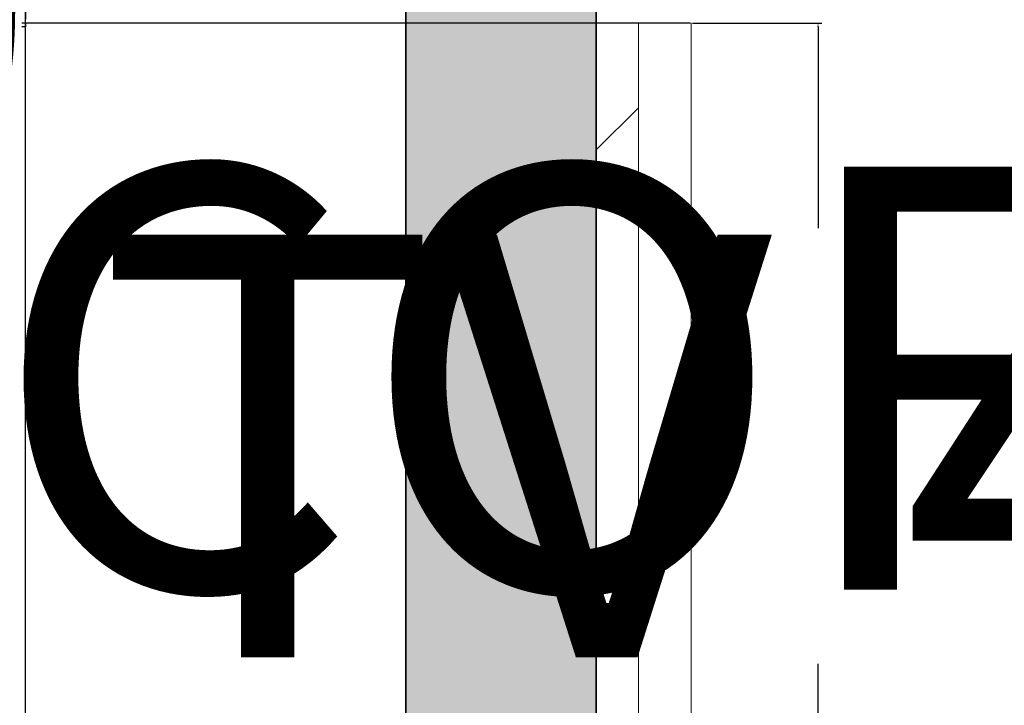
# Model space of a CAD drawing. Units: inches. Extents: x 305 to 776, y 38 to 479.
# Tile 4 of 14: x 372 to 419, y 199 to 231. Entities that reach past the tile are written whole.
import ezdxf

# ---------------------------------------------------------------- set-up
doc = ezdxf.new("R2010")
doc.units = ezdxf.units.IN
doc.header["$MEASUREMENT"] = 0
for name, color, linetype, lineweight in [('A-ANNO-DIMS', 2, 'Continuous', 18), ('A-EQPM', 8, 'Continuous', 18), ('A-WALL', 7, 'Continuous', 35), ('A-WALL-PATT', 252, 'Continuous', 13)]:
    doc.layers.add(name, color=color, linetype=linetype, lineweight=lineweight)
doc.styles.get("Standard").update_dxf_attribs({"font": 'arial.ttf'})
doc.dimstyles.get("Standard").update_dxf_attribs({"dimtxt": 20, "dimasz": 0.18, "dimexe": 0.18, "dimexo": 0.0625, "dimgap": 0.09, "dimtad": 0, "dimtih": 1, "dimtoh": 1, "dimdec": 4, "dimzin": 0, "dimdsep": 46, "dimtxsty": 'Standard', "dimcen": 0.09, "dimadec": 0, "dimazin": 0, "dimtfac": 1, "dimtdec": 4, "dimtofl": 0, "dimtmove": 0, "dimatfit": 3, "dimfxl": 1, "dimtolj": 1, "dimtzin": 0, "dimarcsym": 0})

# ---------------------------------------------------------------- blocks, each defined once
blk = doc.blocks.new('TV')
for p, q in [((722.63, 295.634), (720.13, 295.634)), ((720.13, 295.634), (720.13, 255.634)), ((722.63, 255.634), (722.63, 295.634)), ((720.13, 291.634), (718.13, 289.634)), ((718.13, 289.634), (718.13, 261.634)), ((720.13, 259.634), (718.13, 261.634)), ((720.13, 255.634), (722.63, 255.634))]:
    blk.add_line(p, q)
blk = doc.blocks.new('*D19')
at = {"layer": 'A-ANNO-DIMS', "color": 0, "lineweight": -2, "transparency": 16777216}
for p, q in [((557.633, 250.82), (557.633, 245.977)), ((589.133, 250.82), (589.133, 245.977)), ((557.633, 246.157), (557.453, 246.157)), ((588.953, 246.157), (557.813, 246.157))]:
    blk.add_line(p, q, dxfattribs=at)
at = {"layer": 'A-ANNO-DIMS', "color": 0, "transparency": 16777216}
for points in [[(557.813, 246.187), (557.813, 246.127), (557.633, 246.157)], [(588.953, 246.187), (588.953, 246.127), (589.133, 246.157)]]:
    blk.add_solid(points, dxfattribs=at)
at = {"layer": 'Defpoints', "color": 0, "transparency": 16777216}
for p in [(557.633, 250.882), (589.133, 250.882), (557.633, 246.157)]:
    blk.add_point(p, dxfattribs=at)
at = {"layer": 'A-ANNO-DIMS', "color": 0, "transparency": 16777216, "insert": (463.393, 246.157), "char_height": 20, "attachment_point": 5}
blk.add_mtext('\\A1;DOOR 32 TYP.', dxfattribs=at)
blk = doc.blocks.new('*D37')
at = {"layer": 'A-ANNO-DIMS', "color": 0, "lineweight": -2, "transparency": 16777216}
for p, q in [((476.346, 237.029), (483.222, 237.029)), ((483.042, 236.849), (483.042, 224.939)), ((483.042, 192.153), (483.042, 204.063)), ((476.346, 191.973), (483.222, 191.973))]:
    blk.add_line(p, q, dxfattribs=at)
at = {"layer": 'A-ANNO-DIMS', "color": 0, "transparency": 16777216}
for points in [[(483.012, 236.849), (483.072, 236.849), (483.042, 237.029)], [(483.012, 192.153), (483.072, 192.153), (483.042, 191.973)]]:
    blk.add_solid(points, dxfattribs=at)
at = {"layer": 'Defpoints', "color": 0, "transparency": 16777216}
for p in [(476.283, 237.029), (483.042, 237.029), (476.283, 191.973)]:
    blk.add_point(p, dxfattribs=at)
at = {"layer": 'A-ANNO-DIMS', "color": 0, "transparency": 16777216, "insert": (483.042, 214.501), "char_height": 20, "attachment_point": 5}
blk.add_mtext('\\A1;COFFEE TABLE 45', dxfattribs=at)
blk = doc.blocks.new('*D39')
at = {"layer": 'A-ANNO-DIMS', "color": 0, "lineweight": -2, "transparency": 16777216}
for p, q in [((404.195, 231.292), (410.313, 231.292)), ((410.133, 231.112), (410.133, 221.593)), ((410.133, 191.472), (410.133, 200.99)), ((404.195, 191.292), (410.313, 191.292))]:
    blk.add_line(p, q, dxfattribs=at)
at = {"layer": 'A-ANNO-DIMS', "color": 0, "transparency": 16777216}
for points in [[(410.103, 231.112), (410.163, 231.112), (410.133, 231.292)], [(410.103, 191.472), (410.163, 191.472), (410.133, 191.292)]]:
    blk.add_solid(points, dxfattribs=at)
at = {"layer": 'Defpoints', "color": 0, "transparency": 16777216}
for p in [(404.133, 231.292), (410.133, 231.292), (404.133, 191.292)]:
    blk.add_point(p, dxfattribs=at)
at = {"layer": 'A-ANNO-DIMS', "color": 0, "transparency": 16777216, "insert": (410.133, 211.292), "char_height": 20, "attachment_point": 5}
blk.add_mtext('\\A1;TV 40', dxfattribs=at)
blk = doc.blocks.new('*D46')
at = {"layer": 'A-ANNO-DIMS', "color": 0, "lineweight": -2, "transparency": 16777216}
for p, q in [((390.57, 429.382), (372.451, 429.382)), ((372.631, 429.202), (372.631, 259.69)), ((372.631, 69.562), (372.631, 239.074)), ((390.57, 69.382), (372.451, 69.382))]:
    blk.add_line(p, q, dxfattribs=at)
at = {"layer": 'A-ANNO-DIMS', "color": 0, "transparency": 16777216}
for points in [[(372.601, 429.202), (372.661, 429.202), (372.631, 429.382)], [(372.601, 69.562), (372.661, 69.562), (372.631, 69.382)]]:
    blk.add_solid(points, dxfattribs=at)
at = {"layer": 'Defpoints', "color": 0, "transparency": 16777216}
for p in [(372.631, 429.382), (390.633, 429.382), (390.633, 69.382)]:
    blk.add_point(p, dxfattribs=at)
at = {"layer": 'A-ANNO-DIMS', "color": 0, "transparency": 16777216, "insert": (372.631, 249.382), "char_height": 20, "attachment_point": 5}
blk.add_mtext('\\A1;360', dxfattribs=at)
blk = doc.blocks.new('*D62')
at = {"layer": 'A-ANNO-DIMS', "color": 0, "lineweight": -2, "transparency": 16777216}
for p, q in [((399.633, 336.32), (399.633, 51.201)), ((423.233, 336.32), (423.233, 51.201)), ((399.813, 51.381), (423.053, 51.381)), ((423.233, 51.381), (423.413, 51.381))]:
    blk.add_line(p, q, dxfattribs=at)
at = {"layer": 'A-ANNO-DIMS', "color": 0, "transparency": 16777216}
for points in [[(399.813, 51.411), (399.813, 51.351), (399.633, 51.381)], [(423.053, 51.411), (423.053, 51.351), (423.233, 51.381)]]:
    blk.add_solid(points, dxfattribs=at)
at = {"layer": 'Defpoints', "color": 0, "transparency": 16777216}
for p in [(399.633, 336.382), (423.233, 336.382), (423.233, 51.381)]:
    blk.add_point(p, dxfattribs=at)
at = {"layer": 'A-ANNO-DIMS', "color": 0, "transparency": 16777216, "insert": (449.642, 51.381), "char_height": 20, "attachment_point": 5}
blk.add_mtext('\\A1;23.6', dxfattribs=at)
blk = doc.blocks.new('*D65')
at = {"layer": 'A-ANNO-DIMS', "color": 0, "lineweight": -2, "transparency": 16777216}
for p, q in [((399.633, 351.219), (399.633, 51.201)), ((421.89, 351.219), (421.89, 51.201)), ((399.813, 51.381), (421.71, 51.381)), ((421.89, 51.381), (422.07, 51.381))]:
    blk.add_line(p, q, dxfattribs=at)
at = {"layer": 'A-ANNO-DIMS', "color": 0, "transparency": 16777216}
for points in [[(399.813, 51.411), (399.813, 51.351), (399.633, 51.381)], [(421.71, 51.411), (421.71, 51.351), (421.89, 51.381)]]:
    blk.add_solid(points, dxfattribs=at)
at = {"layer": 'Defpoints', "color": 0, "transparency": 16777216}
for p in [(399.633, 351.281), (421.89, 351.281), (421.89, 51.381)]:
    blk.add_point(p, dxfattribs=at)
at = {"layer": 'A-ANNO-DIMS', "color": 0, "transparency": 16777216, "insert": (463.844, 51.381), "char_height": 20, "attachment_point": 5}
blk.add_mtext('\\A1;22.257', dxfattribs=at)
blk = doc.blocks.new('*D74')
at = {"layer": 'A-ANNO-DIMS', "color": 0, "lineweight": -2, "transparency": 16777216}
for p, q in [((399.57, 250.482), (372.451, 250.482)), ((372.631, 250.302), (372.631, 231.472)), ((404.07, 231.292), (372.451, 231.292)), ((372.631, 231.112), (372.451, 231.112)), ((372.631, 231.292), (372.631, 231.112))]:
    blk.add_line(p, q, dxfattribs=at)
at = {"layer": 'A-ANNO-DIMS', "color": 0, "transparency": 16777216}
for points in [[(372.601, 250.302), (372.661, 250.302), (372.631, 250.482)], [(372.601, 231.472), (372.661, 231.472), (372.631, 231.292)]]:
    blk.add_solid(points, dxfattribs=at)
at = {"layer": 'Defpoints', "color": 0, "transparency": 16777216}
for p in [(399.633, 250.482), (372.631, 231.292), (404.133, 231.292)]:
    blk.add_point(p, dxfattribs=at)
at = {"layer": 'A-ANNO-DIMS', "color": 0, "transparency": 16777216, "insert": (339.537, 231.112), "char_height": 20, "attachment_point": 5}
blk.add_mtext('\\A1;19.19', dxfattribs=at)

msp = doc.modelspace()

# ---------------------------------------------------------------- hatches: boundary and pattern name
at = {"layer": 'A-WALL-PATT'}
h = msp.add_hatch(color=256, dxfattribs=at)
h.dxf.hatch_style = 1
h.paths.add_polyline_path([(481.3329, 429.382), (390.6329, 429.382), (390.6329, 398.067), (399.6329, 398.067), (399.6329, 420.382), (465.6329, 420.382), (465.6329, 331.882), (470.1329, 331.882), (470.1329, 355.882), (512.1329, 355.882), (512.1329, 337.282), (512.1329, 337.282), (515.8592, 337.282), (516.6329, 337.282), (516.6329, 360.382), (513.3171, 360.382), (470.1329, 360.382), (470.1329, 420.382), (481.3329, 420.382)])
h.paths.add_polyline_path([(630.6329, 429.382), (500.9329, 429.382), (500.9329, 420.382), (502.8693, 420.382), (512.1329, 420.382), (512.1329, 391.882), (516.6329, 391.882), (516.6329, 420.382), (621.6329, 420.382), (621.6329, 388.182), (630.6329, 388.182)])
h.paths.add_polyline_path([(630.6329, 329.382), (621.6329, 329.382), (621.6329, 301.882), (512.1329, 301.882), (512.1329, 297.382), (515.8592, 297.382), (557.6329, 297.382), (621.6329, 297.382), (621.6329, 286.182), (630.6329, 286.182)])
h.paths.add_polyline_path([(630.6329, 266.582), (621.6329, 266.582), (621.6329, 255.382), (589.1329, 255.382), (589.1329, 250.882), (621.6329, 250.882), (621.6329, 226.282), (630.6329, 226.282)])
h.paths.add_polyline_path([(630.6329, 167.482), (621.6329, 167.482), (621.6329, 149.1444), (621.6329, 142.882), (516.6329, 142.882), (516.6329, 261.982), (512.1329, 261.982), (512.1329, 138.382), (621.6329, 138.382), (621.6329, 78.382), (512.1329, 78.382), (512.1329, 69.382), (630.6329, 69.382)])
h.paths.add_polyline_path([(464.1329, 138.382), (476.7329, 138.382), (476.7329, 142.1084), (476.7329, 142.882), (459.6329, 142.882), (459.6329, 78.382), (399.6329, 78.382), (399.6329, 98.582), (390.6329, 98.582), (390.6329, 69.382), (464.1329, 69.382)])
h.paths.add_polyline_path([(459.6329, 142.882), (439.3329, 142.882), (439.3329, 138.382), (459.6329, 138.382)], flags=17)
h.paths.add_polyline_path([(399.6329, 138.382), (403.9329, 138.382), (403.9329, 141.5545), (403.9329, 141.5545), (403.9329, 142.882), (399.6329, 142.882), (399.6329, 250.4819), (390.6329, 250.4819), (390.6329, 118.182), (399.6329, 118.182)])
h.paths.add_polyline_path([(399.6329, 331.882), (428.2629, 331.882), (428.2629, 336.382), (399.6329, 336.382), (399.6329, 358.697), (390.6329, 358.697), (390.6329, 309.2819), (399.6329, 309.2819)])

# ---------------------------------------------------------------- linework, layer by layer
at = {"layer": 'A-WALL'}
msp.add_line((399.6329, 331.882), (399.6329, 142.882), dxfattribs=at)
msp.add_lwpolyline([(390.6329, 69.382), (630.6329, 69.382), (630.6329, 429.382), (390.6329, 429.382)], close=True, dxfattribs=at)

# ---------------------------------------------------------------- block references
at = {"layer": 'A-EQPM'}
msp.add_blockref('TV', (-318.4969, -64.3429), dxfattribs=at)

# ---------------------------------------------------------------- dimensions: what is measured, and where the dimension line sits
at = {"layer": 'A-ANNO-DIMS'}
for base, p1, p2, override, picture, middle in [((372.6314, 429.382), (390.6329, 69.382), (390.6329, 429.382), {"dimdec": 0, "dimlfac": 1, "dimrnd": 0, "dimzin": 0, "dimdsep": 46, "dimlunit": 2}, '*D46', (372.6314, 249.382)), ((372.6314, 231.2915), (399.6329, 250.4819), (404.1329, 231.2915), {"dimdec": 2, "dimlfac": 1, "dimrnd": 0, "dimzin": 0, "dimdsep": 46, "dimlunit": 2}, '*D74', (339.5374, 231.1115))]:
    dim = msp.add_linear_dim(base=base, p1=p1, p2=p2, angle=90, dimstyle='Standard', override=override, dxfattribs=at)
    dim.commit()
    dim.dimension.update_dxf_attribs({"geometry": picture, "text_midpoint": middle})
for base, p1, p2, override, picture, middle in [((421.8895, 51.3805), (399.6329, 351.2815), (421.8895, 351.2815), {"dimdec": 3, "dimlfac": 1, "dimrnd": 0, "dimzin": 0, "dimdsep": 46, "dimlunit": 2}, '*D65', (463.8444, 51.3805)), ((423.2329, 51.3805), (399.6329, 336.382), (423.2329, 336.382), {"dimdec": 1, "dimlfac": 1, "dimrnd": 0, "dimzin": 0, "dimdsep": 46, "dimlunit": 2}, '*D62', (449.6421, 51.3805))]:
    dim = msp.add_linear_dim(base=base, p1=p1, p2=p2, dimstyle='Standard', override=override, dxfattribs=at)
    dim.commit()
    dim.dimension.update_dxf_attribs({"geometry": picture, "text_midpoint": middle})
for base, p1, p2, angle, text, picture, middle in [((557.6329062952, 246.15704135), (589.1329062952, 250.88204135), (557.6329062952, 250.88204135), 180, 'DOOR <> TYP.', '*D19', (463.3929199378, 246.15704135)), ((483.0416, 237.0288), (476.2832, 191.9726), (476.2832, 237.0288), 90, 'COFFEE TABLE <>', '*D37', (483.0416, 214.5007)), ((410.1329, 231.2915), (404.1329, 191.2915), (404.1329, 231.2915), 90, 'TV <>', '*D39', (410.1329, 211.2915))]:
    dim = msp.add_linear_dim(base=base, p1=p1, p2=p2, angle=angle, text=text, dimstyle='Standard', override={"dimdec": 0, "dimlfac": 1, "dimrnd": 0, "dimzin": 0, "dimdsep": 46, "dimlunit": 2}, dxfattribs=at)
    dim.commit()
    dim.dimension.update_dxf_attribs({"geometry": picture, "text_midpoint": middle})

doc.saveas('drawing.dxf')
